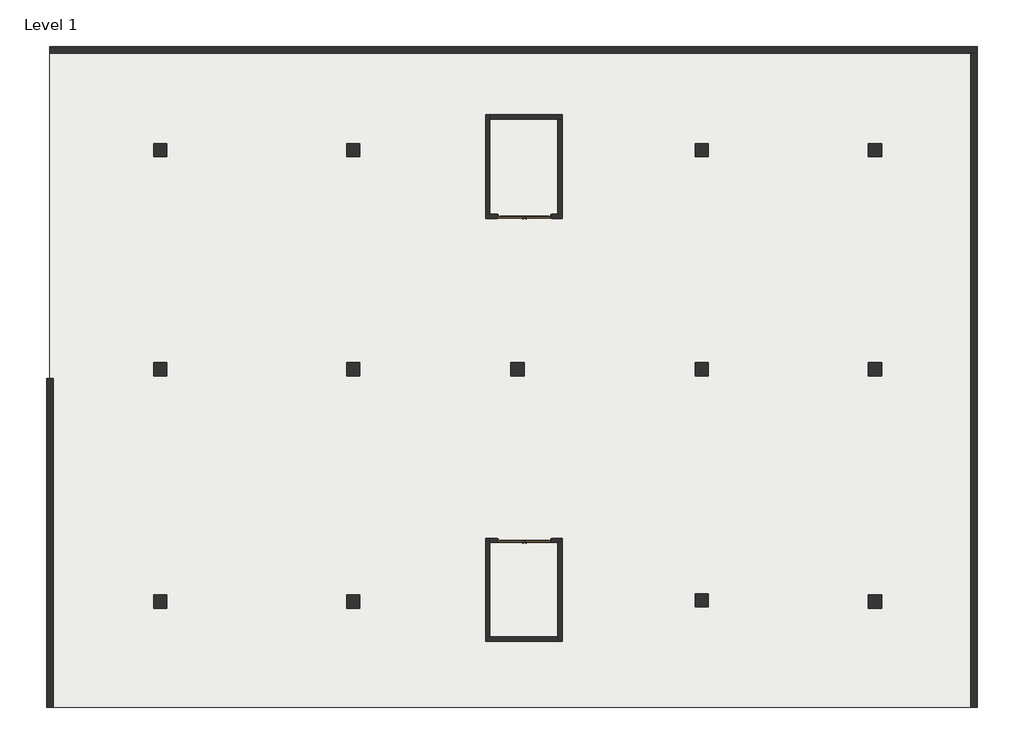
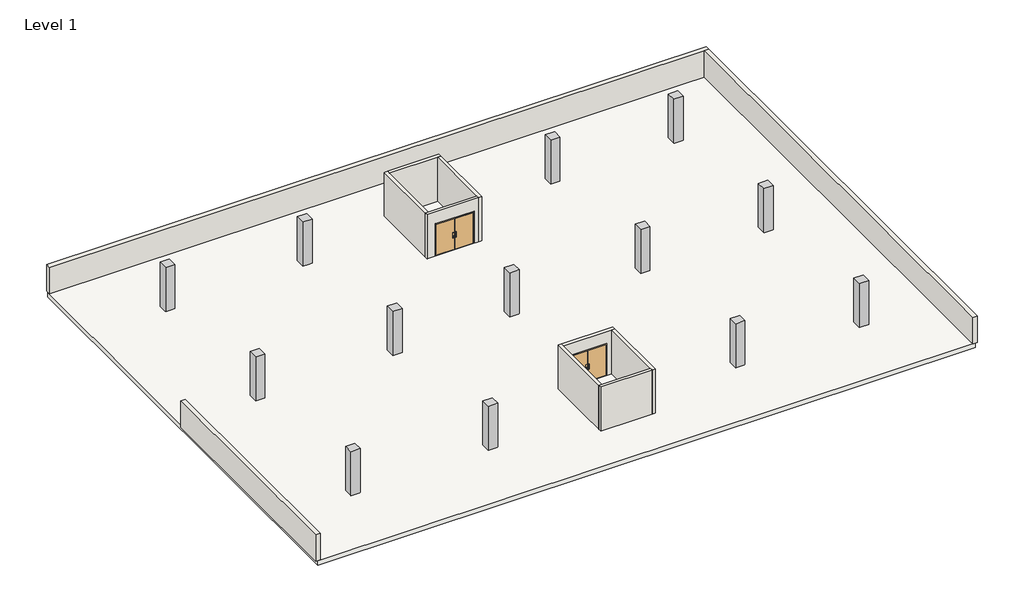
# One storey: 13 columns, 11 walls, 2 doors, 1 slab.
"""IFC4 building model written with IfcOpenShell, lengths in millimetres."""

from ifc_helpers import new_model, si_unit, frame, origin, origin_with_axes, place, context, project, spatial, polyline, outline, extrude, faceted_brep, transform, mapped, element, save
from components import column_c091e905, door_9521ecb0

model = new_model("IFC4")

# Units and contexts
model_context = context("Model", 3, world=origin())
ifc_project = project(units=[si_unit("LENGTHUNIT", "METRE", prefix="MILLI")], contexts=[model_context])

# Site, building, storey
site = spatial("IfcSite", under=ifc_project)
building = spatial("IfcBuilding", under=site)
storey = spatial("IfcBuildingStorey", under=building, Name="Level 1", Elevation=0.0)

# Columns
placement = place(None, origin())
element("IfcColumn", 1, ObjectType="Rectangular Column.0001 : 24\" x 24\"", at=placement, inside=storey, context=model_context, shape_type="SweptSolid", body=[
    extrude(outline(polyline([(-12894.6166248, 14663.4679755), (-12894.6166248, 14053.8679755), (-13504.2166248, 14053.8679755), (-13504.2166248, 14663.4679755), (-12894.6166248, 14663.4679755)])), origin_with_axes(), (0.0, 0.0, 1.0), 3048.0),
])
element("IfcColumn", 2, ObjectType="Rectangular Column.0001 : 24\" x 24\"", at=placement, inside=storey, context=model_context, shape_type="SweptSolid", body=[
    extrude(outline(polyline([(20226.9833752, 14663.4679755), (20226.9833752, 14053.8679755), (19617.3833752, 14053.8679755), (19617.3833752, 14663.4679755), (20226.9833752, 14663.4679755)])), origin_with_axes(), (0.0, 0.0, 1.0), 3048.0),
])
element("IfcColumn", 3, ObjectType="Rectangular Column.0001 : 24\" x 24\"", at=placement, inside=storey, context=model_context, shape_type="SweptSolid", body=[
    extrude(outline(polyline([(20226.9833752, -6266.1320245), (20226.9833752, -6875.7320245), (19617.3833752, -6875.7320245), (19617.3833752, -6266.1320245), (20226.9833752, -6266.1320245)])), origin_with_axes(), (0.0, 0.0, 1.0), 3048.0),
])
element("IfcColumn", 4, ObjectType="Rectangular Column.0001 : 24\" x 24\"", at=placement, inside=storey, context=model_context, shape_type="SweptSolid", body=[
    extrude(outline(polyline([(-12894.6166248, -6266.1320245), (-12894.6166248, -6875.7320245), (-13504.2166248, -6875.7320245), (-13504.2166248, -6266.1320245), (-12894.6166248, -6266.1320245)])), origin_with_axes(), (0.0, 0.0, 1.0), 3048.0),
])
element("IfcColumn", 5, ObjectType="Rectangular Column.0001 : 24\" x 24\"", at=placement, inside=storey, context=model_context, shape_type="SweptSolid", body=[
    extrude(outline(polyline([(-12894.6166248, 4503.4679755), (-12894.6166248, 3893.8679755), (-13504.2166248, 3893.8679755), (-13504.2166248, 4503.4679755), (-12894.6166248, 4503.4679755)])), origin_with_axes(), (0.0, 0.0, 1.0), 3048.0),
])
element("IfcColumn", 6, ObjectType="Rectangular Column.0001 : 24\" x 24\"", at=placement, inside=storey, context=model_context, shape_type="SweptSolid", body=[
    extrude(outline(polyline([(20226.9833752, 4503.4679755), (20226.9833752, 3893.8679755), (19617.3833752, 3893.8679755), (19617.3833752, 4503.4679755), (20226.9833752, 4503.4679755)])), origin_with_axes(), (0.0, 0.0, 1.0), 3048.0),
])
element("IfcColumn", 7, ObjectType="Rectangular Column.0001 : 24\" x 24\"", at=placement, inside=storey, context=model_context, shape_type="SweptSolid", body=[
    extrude(outline(polyline([(12200.5833752, 14663.4679755), (12200.5833752, 14053.8679755), (11590.9833752, 14053.8679755), (11590.9833752, 14663.4679755), (12200.5833752, 14663.4679755)])), origin_with_axes(), (0.0, 0.0, 1.0), 3048.0),
])
element("IfcColumn", 8, ObjectType="Rectangular Column.0001 : 24\" x 24\"", at=placement, inside=storey, context=model_context, shape_type="SweptSolid", body=[
    extrude(outline(polyline([(12200.5833752, -6215.3320245), (12200.5833752, -6824.9320245), (11590.9833752, -6824.9320245), (11590.9833752, -6215.3320245), (12200.5833752, -6215.3320245)])), origin_with_axes(), (0.0, 0.0, 1.0), 3048.0),
])
element("IfcColumn", 9, ObjectType="Rectangular Column.0001 : 24\" x 24\"", at=placement, inside=storey, context=model_context, shape_type="SweptSolid", body=[
    extrude(outline(polyline([(-3953.8166248, 14663.4679755), (-3953.8166248, 14053.8679755), (-4563.4166248, 14053.8679755), (-4563.4166248, 14663.4679755), (-3953.8166248, 14663.4679755)])), origin_with_axes(), (0.0, 0.0, 1.0), 3048.0),
])
element("IfcColumn", 10, ObjectType="Rectangular Column.0001 : 24\" x 24\"", at=placement, inside=storey, context=model_context, shape_type="SweptSolid", body=[
    extrude(outline(polyline([(-3953.8166248, -6266.1320245), (-3953.8166248, -6875.7320245), (-4563.4166248, -6875.7320245), (-4563.4166248, -6266.1320245), (-3953.8166248, -6266.1320245)])), origin_with_axes(), (0.0, 0.0, 1.0), 3048.0),
])
column_shape = column_c091e905(model_context)
element("IfcColumn", 11, ObjectType="Rectangular Column.0001 : 24\" x 24\"", at=placement, inside=storey, context=model_context, shape_type="MappedRepresentation", body=[
    mapped(column_shape, transform((3361.3833752, 4198.6679755, 0.0), x_axis=(1.0, 0.0, 0.0), y_axis=(0.0, 1.0, 0.0), z_axis=(0.0, 0.0, 1.0))),
])
element("IfcColumn", 12, ObjectType="Rectangular Column.0001 : 24\" x 24\"", at=placement, inside=storey, context=model_context, shape_type="MappedRepresentation", body=[
    mapped(column_shape, transform((-4258.6166248, 4198.6679755, 0.0), x_axis=(1.0, 0.0, 0.0), y_axis=(0.0, 1.0, 0.0), z_axis=(0.0, 0.0, 1.0))),
])
element("IfcColumn", 13, ObjectType="Rectangular Column.0001 : 24\" x 24\"", at=placement, inside=storey, context=model_context, shape_type="MappedRepresentation", body=[
    mapped(column_shape, transform((11895.7833752, 4198.6679755, 0.0), x_axis=(1.0, 0.0, 0.0), y_axis=(0.0, 1.0, 0.0), z_axis=(0.0, 0.0, 1.0))),
])

# Doors
door_shape = door_9521ecb0(model_context)
element("IfcDoor", 14, ObjectType="Door-Exterior-Double : 96\" x 84\"", at=placement, inside=storey, context=model_context, shape_type="MappedRepresentation", body=[
    mapped(door_shape, transform((3685.4562622, -3731.1961695, 0.0), x_axis=(-1.0, 0.0, 0.0), y_axis=(0.0, -1.0, 0.0), z_axis=(0.0, 0.0, 1.0))),
])
element("IfcDoor", 15, ObjectType="Door-Exterior-Double : 96\" x 84\"", at=placement, inside=storey, context=model_context, shape_type="MappedRepresentation", body=[
    mapped(door_shape, transform((3685.4562622, 11293.2205944, 0.0), x_axis=(-1.0, 0.0, 0.0), y_axis=(0.0, -1.0, 0.0), z_axis=(0.0, 0.0, 1.0))),
])

# Slab
element("IfcSlab", 16, ObjectType="Generic - 12\"", at=placement, inside=storey, context=model_context, shape_type="SweptSolid", body=[
    extrude(outline(polyline([(24515.5355971, 19008.1538305), (24515.5355971, -11471.8461695), (-18308.8644029, -11471.8461695), (-18308.8644029, 19008.1538305), (24515.5355971, 19008.1538305)])), frame((0.0, 0.0, -304.8), z_axis=(0.0, 0.0, 1.0), x_axis=(1.0, 0.0, 0.0)), (0.0, 0.0, 1.0), 304.8),
])

# Walls
element("IfcWall", 17, ObjectType="Generic - 2'", at=placement, inside=storey, context=model_context, shape_type="Brep", body=[
    faceted_brep([(-18308.8644029, 18855.7538305, 0.0), (24363.1355971, 18855.7538305, 0.0), (24667.9355971, 18855.7538305, 0.0), (24667.9355971, 18855.7538305, 1828.8), (24363.1355971, 18855.7538305, 1828.8), (-18308.8644029, 18855.7538305, 1828.8), (-18308.8644029, 19160.5538305, 0.0), (-18308.8644029, 19160.5538305, 1828.8), (24667.9355971, 19160.5538305, 1828.8), (24667.9355971, 19160.5538305, 0.0)], [[[0, 1, 2, 3, 4, 5]], [[6, 7, 8, 9]], [[2, 1, 0, 6, 9]], [[5, 4, 3, 8, 7]], [[0, 5, 7, 6]], [[3, 2, 9, 8]]]),
])
element("IfcWall", 18, ObjectType="Generic - 2'", at=placement, inside=storey, context=model_context, shape_type="SweptSolid", body=[
    extrude(outline(polyline([(24363.1355971, -11471.8461695), (24363.1355971, 18855.7538305), (24667.9355971, 18855.7538305), (24667.9355971, -11471.8461695), (24363.1355971, -11471.8461695)])), origin_with_axes(), (0.0, 0.0, 1.0), 1828.8),
])
element("IfcWall", 19, ObjectType="Generic - 2'", at=placement, inside=storey, context=model_context, shape_type="SweptSolid", body=[
    extrude(outline(polyline([(-18156.4644029, 3768.1538305), (-18156.4644029, -11471.8461695), (-18461.2644029, -11471.8461695), (-18461.2644029, 3768.1538305), (-18156.4644029, 3768.1538305)])), origin_with_axes(), (0.0, 0.0, 1.0), 1828.8),
])
element("IfcWall", 20, ObjectType="Generic - 8\" white", at=placement, inside=storey, context=model_context, shape_type="Brep", body=[
    faceted_brep([(1880.2520665, -8411.1461695, 0.0), (5233.0520665, -8411.1461695, 0.0), (5233.0520665, -8411.1461695, 3048.0), (1880.2520665, -8411.1461695, 3048.0), (1880.2520665, -8207.9461695, 0.0), (1880.2520665, -8207.9461695, 3048.0), (2083.4520665, -8207.9461695, 3048.0), (5233.0520665, -8207.9461695, 3048.0), (5233.0520665, -8207.9461695, 0.0), (2083.4520665, -8207.9461695, 0.0)], [[[0, 1, 2, 3]], [[4, 5, 6, 7, 8, 9]], [[1, 0, 4, 9, 8]], [[3, 2, 7, 6, 5]], [[0, 3, 5, 4]], [[2, 1, 8, 7]]]),
])
element("IfcWall", 21, ObjectType="Generic - 8\" white", at=placement, inside=storey, context=model_context, shape_type="Brep", body=[
    faceted_brep([(1880.2520665, -3635.9461695, 0.0), (1880.2520665, -8207.9461695, 0.0), (1880.2520665, -8207.9461695, 3048.0), (1880.2520665, -3635.9461695, 3048.0), (2083.4520665, -3635.9461695, 0.0), (2083.4520665, -3635.9461695, 3048.0), (2083.4520665, -3839.1461695, 3048.0), (2083.4520665, -8207.9461695, 3048.0), (2083.4520665, -8207.9461695, 0.0), (2083.4520665, -3839.1461695, 0.0)], [[[0, 1, 2, 3]], [[4, 5, 6, 7, 8, 9]], [[1, 0, 4, 9, 8]], [[3, 2, 7, 6, 5]], [[0, 3, 5, 4]], [[2, 1, 8, 7]]]),
])
element("IfcWall", 22, ObjectType="Generic - 8\" white", at=placement, inside=storey, context=model_context, shape_type="Brep", body=[
    faceted_brep([(2083.4520665, -3635.9461695, 3048.0), (5436.2520665, -3635.9461695, 3048.0), (5436.2520665, -3635.9461695, 0.0), (4955.4562622, -3635.9461695, 0.0), (4955.4562622, -3635.9461695, 2235.2), (2415.4562622, -3635.9461695, 2235.2), (2415.4562622, -3635.9461695, 0.0), (2083.4520665, -3635.9461695, 0.0), (5436.2520665, -3839.1461695, 3048.0), (5233.0520665, -3839.1461695, 3048.0), (2083.4520665, -3839.1461695, 3048.0), (2083.4520665, -3839.1461695, 0.0), (2415.4562622, -3839.1461695, 0.0), (2415.4562622, -3839.1461695, 2235.2), (4955.4562622, -3839.1461695, 2235.2), (4955.4562622, -3839.1461695, 0.0), (5233.0520665, -3839.1461695, 0.0), (5436.2520665, -3839.1461695, 0.0)], [[[0, 1, 2, 3, 4, 5, 6, 7]], [[8, 9, 10, 11, 12, 13, 14, 15, 16, 17]], [[2, 17, 16, 15, 3]], [[11, 7, 6, 12]], [[1, 0, 10, 9, 8]], [[2, 1, 8, 17]], [[0, 7, 11, 10]], [[5, 13, 12, 6]], [[13, 5, 4, 14]], [[14, 4, 3, 15]]]),
])
element("IfcWall", 23, ObjectType="Generic - 8\" white", at=placement, inside=storey, context=model_context, shape_type="Brep", body=[
    faceted_brep([(5436.2520665, -8411.1461695, 0.0), (5436.2520665, -3839.1461695, 0.0), (5436.2520665, -3839.1461695, 3048.0), (5436.2520665, -8411.1461695, 3048.0), (5233.0520665, -8411.1461695, 0.0), (5233.0520665, -8411.1461695, 3048.0), (5233.0520665, -8207.9461695, 3048.0), (5233.0520665, -3839.1461695, 3048.0), (5233.0520665, -3839.1461695, 0.0), (5233.0520665, -8207.9461695, 0.0)], [[[0, 1, 2, 3]], [[4, 5, 6, 7, 8, 9]], [[1, 0, 4, 9, 8]], [[3, 2, 7, 6, 5]], [[0, 3, 5, 4]], [[2, 1, 8, 7]]]),
])
element("IfcWall", 24, ObjectType="Generic - 8\" white", at=placement, inside=storey, context=model_context, shape_type="Brep", body=[
    faceted_brep([(5436.2520665, 15993.8548886, 0.0), (2083.4520665, 15993.8548886, 0.0), (2083.4520665, 15993.8548886, 3048.0), (5436.2520665, 15993.8548886, 3048.0), (5436.2520665, 15790.6548886, 0.0), (5436.2520665, 15790.6548886, 3048.0), (5233.0520665, 15790.6548886, 3048.0), (2083.4520665, 15790.6548886, 3048.0), (2083.4520665, 15790.6548886, 0.0), (5233.0520665, 15790.6548886, 0.0)], [[[0, 1, 2, 3]], [[4, 5, 6, 7, 8, 9]], [[1, 0, 4, 9, 8]], [[3, 2, 7, 6, 5]], [[0, 3, 5, 4]], [[2, 1, 8, 7]]]),
])
element("IfcWall", 25, ObjectType="Generic - 8\" white", at=placement, inside=storey, context=model_context, shape_type="Brep", body=[
    faceted_brep([(5436.2520665, 11185.2705944, 0.0), (5436.2520665, 15790.6548886, 0.0), (5436.2520665, 15790.6548886, 3048.0), (5436.2520665, 11185.2705944, 3048.0), (5233.0520665, 11185.2705944, 0.0), (5233.0520665, 11185.2705944, 3048.0), (5233.0520665, 11388.4705944, 3048.0), (5233.0520665, 15790.6548886, 3048.0), (5233.0520665, 15790.6548886, 0.0), (5233.0520665, 11388.4705944, 0.0)], [[[0, 1, 2, 3]], [[4, 5, 6, 7, 8, 9]], [[1, 0, 4, 9, 8]], [[3, 2, 7, 6, 5]], [[0, 3, 5, 4]], [[2, 1, 8, 7]]]),
])
element("IfcWall", 26, ObjectType="Generic - 8\" white", at=placement, inside=storey, context=model_context, shape_type="Brep", body=[
    faceted_brep([(5233.0520665, 11185.2705944, 3048.0), (1880.2520665, 11185.2705944, 3048.0), (1880.2520665, 11185.2705944, 0.0), (2415.4562622, 11185.2705944, 0.0), (2415.4562622, 11185.2705944, 2235.2), (4955.4562622, 11185.2705944, 2235.2), (4955.4562622, 11185.2705944, 0.0), (5233.0520665, 11185.2705944, 0.0), (1880.2520665, 11388.4705944, 3048.0), (2083.4520665, 11388.4705944, 3048.0), (5233.0520665, 11388.4705944, 3048.0), (5233.0520665, 11388.4705944, 0.0), (4955.4562622, 11388.4705944, 0.0), (4955.4562622, 11388.4705944, 2235.2), (2415.4562622, 11388.4705944, 2235.2), (2415.4562622, 11388.4705944, 0.0), (2083.4520665, 11388.4705944, 0.0), (1880.2520665, 11388.4705944, 0.0)], [[[0, 1, 2, 3, 4, 5, 6, 7]], [[8, 9, 10, 11, 12, 13, 14, 15, 16, 17]], [[2, 17, 16, 15, 3]], [[11, 7, 6, 12]], [[1, 0, 10, 9, 8]], [[2, 1, 8, 17]], [[0, 7, 11, 10]], [[14, 4, 3, 15]], [[4, 14, 13, 5]], [[5, 13, 12, 6]]]),
])
element("IfcWall", 27, ObjectType="Generic - 8\" white", at=placement, inside=storey, context=model_context, shape_type="Brep", body=[
    faceted_brep([(1880.2520665, 15993.8548886, 0.0), (1880.2520665, 11388.4705944, 0.0), (1880.2520665, 11388.4705944, 3048.0), (1880.2520665, 15993.8548886, 3048.0), (2083.4520665, 15993.8548886, 0.0), (2083.4520665, 15993.8548886, 3048.0), (2083.4520665, 15790.6548886, 3048.0), (2083.4520665, 11388.4705944, 3048.0), (2083.4520665, 11388.4705944, 0.0), (2083.4520665, 15790.6548886, 0.0)], [[[0, 1, 2, 3]], [[4, 5, 6, 7, 8, 9]], [[1, 0, 4, 9, 8]], [[3, 2, 7, 6, 5]], [[0, 3, 5, 4]], [[2, 1, 8, 7]]]),
])

save(model, "model.ifc")

# Revit data of these elements
# Type "Rectangular Column.0001 : 24\" x 24\""
#   Assembly Code = "B1010200"
#   Depth = 2' - 0"
#   Offset Base = 0' - 0"
#   Offset Top = 0' - 0"
#   Width = 2' - 0"
#   Material = Metal - Painted - Grey
# Type "Door-Exterior-Double : 96\" x 84\""
#   Type Mark = "11"
#   Assembly Code = "B2030200"
#   Analytic Construction = "Metal"
#   Threshold Length [instance default] = 8' - 4"
#   Threshold Offset [instance default] = 0' - 0 1/2"
#   Thickness = 0' - 1 3/4"
#   Thermal Resistance (R) = 1.5338 (h·ft²·°F)/BTU
#   Swing Angle [instance default] = 90.00°
#   Strike Height = 3' - 4"
#   SinglePanelWidth = 4' - 0"
#   Rough Width [instance default] = 8' - 4"
#   Rough Height [instance default] = 7' - 4"
#   MFOpeningHeight [instance default] = 0' - 4"
#   MFOpeningWidth [instance default] = 0' - 4"
#   Inset Calculate [instance default] = 0' - 4"
#   Masonry Inset [instance default] = 0' - 1"
#   Height = 7' - 0"
#   Width = 8' - 0"
#   Heat Transfer Coefficient (U) = 0.6520 BTU/(h·ft²·°F)
#   Masonry Frame Depth = 0' - 5 3/4"
#   Threshold [instance default] = yes
#   Masonry Frame [instance default] = yes
#   Function = 1
#   Dry Wall Frame [instance default] = no
#   Threshold Material = Cherry
#   Panic Bar Material = Metal - Stainless Steel
#   Panel Material = Metal - Painted - Grey
#   Frame Material = Metal - Painted - Grey
#   Exterior Pull Material = Metal - Stainless Steel
#   Visual Light Transmittance = 0
#   Solar Heat Gain Coefficient = 0
#   Wall Closure = (empty or 0)
# Type "Generic - 12\""
#   Assembly Code = "B1010"
#   Function = 0
#   Layers, outside or top first: 1' - 0" "Brick, Soldier Course" (function 1)
# Type "Generic - 2'"
#   Assembly Code = "B2010"
#   Layers, outside or top first: 1' - 0" "Metal - Painted - Grey" (function 1)
# Type "Generic - 8\" white"
#   Assembly Code = "B2010"
#   Layers, outside or top first: 0' - 8" "Metal - Painted - Grey" (function 1)
# Elements 1, 2, 3, 4, 5, 6, 7, 8, 9, 10, 11, 12, 13 (IfcColumn, "Rectangular Column.0001 : 24\" x 24\"")
#   Phase Created = New Construction
#   Materials on its faces: "Metal - Painted - Grey"
# Elements 14, 15 (IfcDoor, "Door-Exterior-Double : 96\" x 84\"")
#   Threshold Offset = 0' - 0 1/2"
#   Threshold Length = 8' - 4"
#   Swing Angle = 90.00°
#   Rough Width = 8' - 4"
#   Rough Height = 7' - 4"
#   Masonry Inset = 0' - 1"
#   MFOpeningWidth = 0' - 4"
#   MFOpeningHeight = 0' - 4"
#   Inset Calculate = 0' - 4"
#   Threshold = yes
#   Masonry Frame = yes
#   Dry Wall Frame = no
#   Phase Created = New Construction
#   Materials on its faces: "Metal - Stainless Steel", "Metal - Painted - Grey", "Cherry"
# Element 16 (IfcSlab, "Generic - 12\"")
#   Height Offset From Level = 0' - 0"
#   Phase Created = New Construction
#   Materials on its faces: "Brick, Soldier Course"
# Elements 17, 18, 19 (IfcWall, "Generic - 2'")
#   Top Offset = 0' - 0"
#   Base Offset = 0' - 0"
#   Unconnected Height = 6' - 0"
#   wall height = 6' - 0"
#   Phase Created = New Construction
#   Base Constraint = Level 1
#   Materials on its faces: "Metal - Painted - Grey"
# Elements 20, 21, 22, 23, 24, 25, 26, 27 (IfcWall, "Generic - 8\" white")
#   Top Offset = 0' - 0"
#   Base Offset = 0' - 0"
#   Unconnected Height = 10' - 0"
#   wall height = 10' - 0"
#   Phase Created = New Construction
#   Base Constraint = Level 1
#   Materials on its faces: "Metal - Painted - Grey"
# Materials
#   "Metal - Painted - Grey": class "Paint", colour RGB 104 104 104, transparency 0, Cost = 0
#   "Cherry": class "Wood", colour RGB 226 177 128, transparency 0, Description = "Prunus Serotina", Cost = 0
#   "Metal - Stainless Steel": class "Metal", colour RGB 247 247 247, transparency 0
#   "Brick, Soldier Course": class "Masonry", colour RGB 170 98 104, transparency 0, Description = "Common brick soldier coursed", Cost = 0
